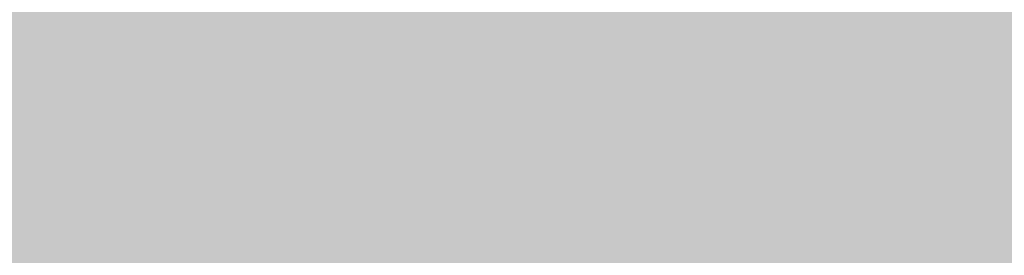
# Model space of a CAD drawing. Units: millimetres. Extents: x 0 to 2267, y 0 to 1823.
# Tile 223 of 256: x 1841.442 to 1842.748, y 1127.462 to 1127.775. Entities that reach past the tile are written whole.
import ezdxf

# ---------------------------------------------------------------- set-up
doc = ezdxf.new("R2010")
doc.units = ezdxf.units.MM
doc.header["$MEASUREMENT"] = 0
doc.layers.add('M-HATC', color=252, linetype='Continuous', lineweight=18)

msp = doc.modelspace()

# ---------------------------------------------------------------- hatches: boundary and pattern name
at = {"layer": 'M-HATC'}
h = msp.add_hatch(color=256, dxfattribs=at)
h.dxf.hatch_style = 1
h.paths.add_polyline_path([(2055.771, 1603.062), (1381.0868, 1603.062), (1381.0868, 1598.062), (2055.771, 1598.062)])
h.paths.add_polyline_path([(2055.771, 1598.062), (1381.0868, 1598.062), (1381.0868, 1593.062), (2055.771, 1593.062)])
h.paths.add_polyline_path([(2051.3074, 1536.7609), (1385.5504, 1536.7609), (1385.5504, 1526.7609), (1387.5504, 1526.7609), (1388.5366, 1525.0528), (1385.3319, 1521.2335), (1385.3319, 1521.2226), (2050.2542, 1522.7491), (2048.3212, 1525.0528), (2049.3074, 1526.7609), (2051.3074, 1526.7609)])
edge = h.paths.add_edge_path()
edge.add_arc((1847.5345, 1379.1492), 135, 222.603061, 222.890851, ccw=False)
edge.add_line((1748.1663, 1287.7656), (1683.0921, 1287.7656))
edge.add_arc((1583.7239, 1379.1492), 135, 317.109149, 317.396939, ccw=False)
edge.add_arc((1678.9686, 1290.6707), 5, 222.8909, 317.1091, ccw=False)
edge.add_arc((1774.2133, 1379.1492), 135, 222.603061, 222.890851, ccw=False)
edge.add_line((1674.8451, 1287.7656), (1609.7709, 1287.7656))
edge.add_arc((1510.4027, 1379.1492), 135, 317.109149, 317.396939, ccw=False)
edge.add_arc((1605.6474, 1290.6707), 5, 222.8909, 317.1091, ccw=False)
edge.add_arc((1700.8921, 1379.1492), 135, 222.603061, 222.890851, ccw=False)
edge.add_line((1601.5239, 1287.7656), (1536.4497, 1287.7656))
edge.add_arc((1437.0815, 1379.1492), 135, 317.109149, 317.396939, ccw=False)
edge.add_arc((1532.3262, 1290.6707), 5, 222.8909, 317.1091, ccw=False)
edge.add_arc((1627.5709, 1379.1492), 135, 222.603061, 222.890851, ccw=False)
edge.add_line((1528.2027, 1287.7656), (1505.9289, 1287.7656))
edge.add_spline(control_points=[(1505.9289, 1287.7656), (1504.2622, 1287.7656), (1504.2622, 1282.7656), (1505.9289, 1282.7656)], knot_values=[0, 0, 0, 0, 5, 5, 5, 5], degree=3, periodic=0)
edge.add_line((1505.9289, 1282.7656), (1930.9289, 1282.7656))
edge.add_spline(control_points=[(1930.9289, 1282.7656), (1932.5956, 1282.7656), (1932.5956, 1287.7656), (1930.9289, 1287.7656)], knot_values=[0, 0, 0, 0, 5, 5, 5, 5], degree=3, periodic=0)
edge.add_line((1930.9289, 1287.7656), (1903.0557, 1287.7656))
edge.add_arc((1803.6875, 1379.1492), 135, 317.109149, 317.396939, ccw=False)
edge.add_arc((1898.9322, 1290.6707), 5, 222.8909, 317.1091, ccw=False)
edge.add_arc((1994.1769, 1379.1492), 135, 222.603061, 222.890851, ccw=False)
edge.add_line((1894.8087, 1287.7656), (1829.7345, 1287.7656))
edge.add_arc((1730.3663, 1379.1492), 135, 317.109149, 317.396939, ccw=False)
edge.add_arc((1825.611, 1290.6707), 5, 222.8909, 317.1091, ccw=False)
edge.add_arc((1920.8557, 1379.1492), 135, 222.603061, 222.890851, ccw=False)
edge.add_line((1821.4875, 1287.7656), (1756.4133, 1287.7656))
edge.add_arc((1657.0451, 1379.1492), 135, 317.109149, 317.396939, ccw=False)
edge.add_arc((1752.2898, 1290.6707), 5, 222.8909, 317.1091, ccw=False)
edge = h.paths.add_edge_path()
edge.add_spline(control_points=[(1843.4289, 1227.2475), (1845.0956, 1227.2475), (1845.0956, 1232.2475), (1843.4289, 1232.2475)], knot_values=[0, 0, 0, 0, 5, 5, 5, 5], degree=3, periodic=0)
edge.add_line((1843.4289, 1232.2475), (1593.4289, 1232.2475))
edge.add_spline(control_points=[(1593.4289, 1232.2475), (1591.7622, 1232.2475), (1591.7622, 1227.2475), (1593.4289, 1227.2475)], knot_values=[0, 0, 0, 0, 5, 5, 5, 5], degree=3, periodic=0)
edge.add_line((1593.4289, 1227.2475), (1843.4289, 1227.2475))
h.paths.add_polyline_path([(1905.9289, 1127.4171), (1530.9289, 1127.4171, 0.414214), (1520.9289, 1117.4171), (1530.9289, 1117.4171), (1915.9289, 1117.4171, 0.414214)])
edge = h.paths.add_edge_path()
edge.add_arc((1397.0858, 1498.4078), 12.7299, 90.78215, 190.87871, ccw=False)
edge.add_line((1396.912, 1511.1365), (1428.0097, 1511.3488))
edge.add_line((1428.0097, 1511.3488), (1433.0097, 1511.3488))
edge.add_line((1433.0097, 1511.3488), (1434.439, 1511.3488))
edge.add_arc((1419.474, 1498.0804), 20, 41.561, 74.08211)
edge.add_line((1424.9592, 1517.3135), (1399.9351, 1517.2561))
edge.add_spline(control_points=[(1399.9307, 1517.2561), (1399.884, 1517.2131), (1399.8328, 1517.1689), (1399.7774, 1517.1236)], knot_values=[11.567499, 11.567499, 11.567499, 11.567499, 11.814249, 11.814249, 11.814249, 11.814249], degree=3, periodic=0)
edge.add_spline(control_points=[(1399.6328, 1517.0099), (1399.5831, 1516.9721), (1399.5307, 1516.9338), (1399.4759, 1516.8947)], knot_values=[11.167718, 11.167718, 11.167718, 11.167718, 11.365188, 11.365188, 11.365188, 11.365188], degree=3, periodic=0)
edge.add_spline(control_points=[(1399.3398, 1516.8001), (1399.1514, 1516.6719), (1398.9384, 1516.5377), (1398.704, 1516.3994)], knot_values=[10.376405, 10.376405, 10.376405, 10.376405, 11.00994, 11.00994, 11.00994, 11.00994], degree=3, periodic=0)
edge.add_spline(control_points=[(1398.6572, 1516.3719), (1398.5789, 1516.326), (1398.4983, 1516.2797), (1398.4155, 1516.2331)], knot_values=[10.125175, 10.125175, 10.125175, 10.125175, 10.334406, 10.334406, 10.334406, 10.334406], degree=3, periodic=0)
edge.add_spline(control_points=[(1398.2642, 1516.1487), (1398.196, 1516.1111), (1398.1263, 1516.0732), (1398.0555, 1516.0351)], knot_values=[9.832246, 9.832246, 9.832246, 9.832246, 9.999658, 9.999658, 9.999658, 9.999658], degree=3, periodic=0)
edge.add_spline(control_points=[(1397.9987, 1516.0048), (1397.7312, 1515.8621), (1397.446, 1515.7171), (1397.1466, 1515.5714)], knot_values=[9.161808, 9.161808, 9.161808, 9.161808, 9.787769, 9.787769, 9.787769, 9.787769], degree=3, periodic=0)
edge.add_spline(control_points=[(1397.1466, 1515.5714), (1396.8418, 1515.423), (1396.5222, 1515.274), (1396.1914, 1515.1262)], knot_values=[8.524455, 8.524455, 8.524455, 8.524455, 9.161808, 9.161808, 9.161808, 9.161808], degree=3, periodic=0)
edge.add_spline(control_points=[(1396.0777, 1515.0756), (1395.9854, 1515.0348), (1395.8922, 1514.994), (1395.7983, 1514.9534)], knot_values=[8.275193, 8.275193, 8.275193, 8.275193, 8.451726, 8.451726, 8.451726, 8.451726], degree=3, periodic=0)
edge.add_spline(control_points=[(1395.6018, 1514.8691), (1395.4997, 1514.8257), (1395.3968, 1514.7824), (1395.2932, 1514.7394)], knot_values=[7.962917, 7.962917, 7.962917, 7.962917, 8.152764, 8.152764, 8.152764, 8.152764], degree=3, periodic=0)
edge.add_spline(control_points=[(1395.2116, 1514.7057), (1394.8278, 1514.5475), (1394.4345, 1514.3929), (1394.0364, 1514.2442)], knot_values=[7.21254, 7.21254, 7.21254, 7.21254, 7.913148, 7.913148, 7.913148, 7.913148], degree=3, periodic=0)
edge.add_spline(control_points=[(1394.0364, 1514.2442), (1393.7076, 1514.1214), (1393.3754, 1514.0027), (1393.0427, 1513.8895)], knot_values=[6.633733, 6.633733, 6.633733, 6.633733, 7.21254, 7.21254, 7.21254, 7.21254], degree=3, periodic=0)
edge.add_spline(control_points=[(1392.8214, 1513.815), (1392.7198, 1513.7812), (1392.6181, 1513.7479), (1392.5166, 1513.7152)], knot_values=[6.328796, 6.328796, 6.328796, 6.328796, 6.505493, 6.505493, 6.505493, 6.505493], degree=3, periodic=0)
edge.add_spline(control_points=[(1392.5166, 1513.7152), (1392.3187, 1513.6515), (1392.1212, 1513.59), (1391.9244, 1513.531)], knot_values=[5.984605, 5.984605, 5.984605, 5.984605, 6.328796, 6.328796, 6.328796, 6.328796], degree=3, periodic=0)
edge.add_spline(control_points=[(1391.7915, 1513.4915), (1391.3122, 1513.3501), (1390.8384, 1513.2239), (1390.3784, 1513.1171)], knot_values=[5.066697, 5.066697, 5.066697, 5.066697, 5.907055, 5.907055, 5.907055, 5.907055], degree=3, periodic=0)
edge.add_spline(control_points=[(1390.3784, 1513.1171), (1390.1797, 1513.071), (1389.9836, 1513.0284), (1389.7907, 1512.9899)], knot_values=[4.70367, 4.70367, 4.70367, 4.70367, 5.066695, 5.066695, 5.066695, 5.066695], degree=3, periodic=0)
edge.add_spline(control_points=[(1389.422, 1512.9204), (1389.2459, 1512.8892), (1389.0729, 1512.8617), (1388.9036, 1512.8381)], knot_values=[4.130571, 4.130571, 4.130571, 4.130571, 4.469816, 4.469816, 4.469816, 4.469816], degree=3, periodic=0)
edge.add_spline(control_points=[(1388.9036, 1512.8381), (1388.591, 1512.7946), (1388.2911, 1512.7644), (1388.0071, 1512.7494)], knot_values=[3.504031, 3.504031, 3.504031, 3.504031, 4.130571, 4.130571, 4.130571, 4.130571], degree=3, periodic=0)
edge.add_spline(control_points=[(1387.9356, 1512.7459), (1387.8538, 1512.7423), (1387.7733, 1512.74), (1387.6944, 1512.739)], knot_values=[3.268866, 3.268866, 3.268866, 3.268866, 3.451164, 3.451164, 3.451164, 3.451164], degree=3, periodic=0)
edge.add_spline(control_points=[(1387.3351, 1512.7443), (1387.2076, 1512.7499), (1387.0847, 1512.7597), (1386.967, 1512.7739)], knot_values=[2.670686, 2.670686, 2.670686, 2.670686, 2.984, 2.984, 2.984, 2.984], degree=3, periodic=0)
edge.add_spline(control_points=[(1386.8327, 1512.7922), (1386.8209, 1512.7941), (1386.8092, 1512.7959), (1386.7975, 1512.7979)], knot_values=[2.516981, 2.516981, 2.516981, 2.516981, 2.549528, 2.549528, 2.549528, 2.549528], degree=3, periodic=0)
edge.add_spline(control_points=[(1386.4526, 1512.8735), (1386.4257, 1512.881), (1386.3993, 1512.889), (1386.3733, 1512.8972)], knot_values=[2.095869, 2.095869, 2.095869, 2.095869, 2.17941, 2.17941, 2.17941, 2.17941], degree=3, periodic=0)
edge.add_spline(control_points=[(1386.0691, 1513.0189), (1386.0634, 1513.0217), (1386.0577, 1513.0246), (1386.052, 1513.0275)], knot_values=[1.72453, 1.72453, 1.72453, 1.72453, 1.745933, 1.745933, 1.745933, 1.745933], degree=3, periodic=0)
edge.add_arc((1399.474, 1498.0804), 20, 131.82432, 180)
edge.add_arc((1630.3336, 1505.5484), 250.9708, 181.705176, 236.427975)
edge.add_arc((1605.3399, 1483.3044), 218.7822, 238.660829, 243.34961)
edge.add_arc((1647.0911, 1510.3592), 262.8986, 183.129836, 237.853442, ccw=False)
h.paths.add_polyline_path([(1406.5369, 1391.9644, 0.149382), (1491.5506, 1296.4418, -0.129517)], flags=17)
edge = h.paths.add_edge_path()
edge.add_arc((2037.3838, 1498.0804), 20, 0, 48.26587)
edge.add_spline(control_points=[(2050.6973, 1513.0052), (2050.6512, 1512.9847), (2050.6034, 1512.9655), (2050.5539, 1512.9477)], knot_values=[1.835652, 1.835652, 1.835652, 1.835652, 2.000781, 2.000781, 2.000781, 2.000781], degree=3, periodic=0)
edge.add_spline(control_points=[(2050.4616, 1512.9166), (2050.479, 1512.9221), (2050.4963, 1512.9277), (2050.5133, 1512.9335)], knot_values=[2.045477, 2.045477, 2.045477, 2.045477, 2.101389, 2.101389, 2.101389, 2.101389], degree=3, periodic=0)
edge.add_spline(control_points=[(2050.129, 1512.8342), (2050.1984, 1512.8473), (2050.2657, 1512.8623), (2050.3308, 1512.8792)], knot_values=[2.237629, 2.237629, 2.237629, 2.237629, 2.435841, 2.435841, 2.435841, 2.435841], degree=3, periodic=0)
edge.add_spline(control_points=[(2050.0946, 1512.8278), (2050.1061, 1512.8299), (2050.1176, 1512.832), (2050.129, 1512.8342)], knot_values=[2.435841, 2.435841, 2.435841, 2.435841, 2.468321, 2.468321, 2.468321, 2.468321], degree=3, periodic=0)
edge.add_spline(control_points=[(2049.7843, 1512.7851), (2049.8552, 1512.7922), (2049.9243, 1512.8008), (2049.9917, 1512.8109)], knot_values=[2.563852, 2.563852, 2.563852, 2.563852, 2.748541, 2.748541, 2.748541, 2.748541], degree=3, periodic=0)
edge.add_spline(control_points=[(2049.4052, 1512.7617), (2049.5364, 1512.7653), (2049.6629, 1512.773), (2049.7843, 1512.7851)], knot_values=[2.748541, 2.748541, 2.748541, 2.748541, 3.064882, 3.064882, 3.064882, 3.064882], degree=3, periodic=0)
edge.add_spline(control_points=[(2049.1698, 1512.7597), (2049.2336, 1512.7591), (2049.2965, 1512.7594), (2049.3584, 1512.7606)], knot_values=[3.102309, 3.102309, 3.102309, 3.102309, 3.2503, 3.2503, 3.2503, 3.2503], degree=3, periodic=0)
edge.add_spline(control_points=[(2048.8573, 1512.7691), (2048.9638, 1512.7638), (2049.068, 1512.7606), (2049.1698, 1512.7597)], knot_values=[3.2503, 3.2503, 3.2503, 3.2503, 3.486069, 3.486069, 3.486069, 3.486069], degree=3, periodic=0)
edge.add_spline(control_points=[(2048.6924, 1512.7789), (2048.3729, 1512.8009), (2048.0345, 1512.8411), (2047.6817, 1512.897)], knot_values=[3.606429, 3.606429, 3.606429, 3.606429, 4.2989, 4.2989, 4.2989, 4.2989], degree=3, periodic=0)
edge.add_spline(control_points=[(2047.6817, 1512.897), (2047.5458, 1512.9185), (2047.4077, 1512.9424), (2047.2678, 1512.9685)], knot_values=[4.2989, 4.2989, 4.2989, 4.2989, 4.565769, 4.565769, 4.565769, 4.565769], degree=3, periodic=0)
edge.add_spline(control_points=[(2047.2678, 1512.9685), (2047.1449, 1512.9914), (2047.0207, 1513.016), (2046.8951, 1513.0422)], knot_values=[4.565769, 4.565769, 4.565769, 4.565769, 4.799971, 4.799971, 4.799971, 4.799971], degree=3, periodic=0)
edge.add_spline(control_points=[(2046.8951, 1513.0422), (2046.5286, 1513.1188), (2046.1513, 1513.209), (2045.7676, 1513.3107)], knot_values=[4.799971, 4.799971, 4.799971, 4.799971, 5.483718, 5.483718, 5.483718, 5.483718], degree=3, periodic=0)
edge.add_spline(control_points=[(2045.7676, 1513.3107), (2045.3724, 1513.4154), (2044.9704, 1513.5322), (2044.5662, 1513.6588)], knot_values=[5.483718, 5.483718, 5.483718, 5.483718, 6.187866, 6.187866, 6.187866, 6.187866], degree=3, periodic=0)
edge.add_spline(control_points=[(2044.5662, 1513.6588), (2044.4149, 1513.7061), (2044.2633, 1513.7549), (2044.1116, 1513.8048)], knot_values=[6.187866, 6.187866, 6.187866, 6.187866, 6.451551, 6.451551, 6.451551, 6.451551], degree=3, periodic=0)
edge.add_spline(control_points=[(2044.1116, 1513.8048), (2043.9967, 1513.8427), (2043.8817, 1513.8813), (2043.7668, 1513.9205)], knot_values=[6.451551, 6.451551, 6.451551, 6.451551, 6.651434, 6.651434, 6.651434, 6.651434], degree=3, periodic=0)
edge.add_spline(control_points=[(2043.7668, 1513.9205), (2043.3716, 1514.0554), (2042.9774, 1514.1979), (2042.5886, 1514.3458)], knot_values=[6.651434, 6.651434, 6.651434, 6.651434, 7.338879, 7.338879, 7.338879, 7.338879], degree=3, periodic=0)
edge.add_spline(control_points=[(2042.5886, 1514.3458), (2042.1643, 1514.5071), (2041.7465, 1514.6749), (2041.3409, 1514.846)], knot_values=[7.338879, 7.338879, 7.338879, 7.338879, 8.089209, 8.089209, 8.089209, 8.089209], degree=3, periodic=0)
edge.add_spline(control_points=[(2041.3409, 1514.846), (2041.1028, 1514.9465), (2040.869, 1515.0481), (2040.6405, 1515.1502)], knot_values=[8.089209, 8.089209, 8.089209, 8.089209, 8.529587, 8.529587, 8.529587, 8.529587], degree=3, periodic=0)
edge.add_spline(control_points=[(2040.51, 1515.2089), (2040.0824, 1515.4022), (2039.6747, 1515.5971), (2039.295, 1515.7894)], knot_values=[8.613818, 8.613818, 8.613818, 8.613818, 9.44571, 9.44571, 9.44571, 9.44571], degree=3, periodic=0)
edge.add_spline(control_points=[(2039.295, 1515.7894), (2039.0618, 1515.9075), (2038.8391, 1516.0246), (2038.6288, 1516.1398)], knot_values=[9.44571, 9.44571, 9.44571, 9.44571, 9.956404, 9.956404, 9.956404, 9.956404], degree=3, periodic=0)
edge.add_spline(control_points=[(2038.6288, 1516.1398), (2038.5187, 1516.2001), (2038.4121, 1516.2598), (2038.309, 1516.3189)], knot_values=[9.956404, 9.956404, 9.956404, 9.956404, 10.223542, 10.223542, 10.223542, 10.223542], degree=3, periodic=0)
edge.add_spline(control_points=[(2038.309, 1516.3189), (2038.2138, 1516.3735), (2038.1216, 1516.4276), (2038.0328, 1516.481)], knot_values=[10.223542, 10.223542, 10.223542, 10.223542, 10.47051, 10.47051, 10.47051, 10.47051], degree=3, periodic=0)
edge.add_spline(control_points=[(2038.0328, 1516.481), (2037.7855, 1516.6296), (2037.5639, 1516.773), (2037.3722, 1516.909)], knot_values=[10.47051, 10.47051, 10.47051, 10.47051, 11.15767, 11.15767, 11.15767, 11.15767], degree=3, periodic=0)
edge.add_spline(control_points=[(2037.3722, 1516.909), (2037.2789, 1516.9752), (2037.1927, 1517.0396), (2037.1142, 1517.102)], knot_values=[11.15767, 11.15767, 11.15767, 11.15767, 11.49227, 11.49227, 11.49227, 11.49227], degree=3, periodic=0)
edge.add_spline(control_points=[(2036.8564, 1517.3259), (2036.9148, 1517.2692), (2036.9814, 1517.2103), (2037.0557, 1517.1492)], knot_values=[11.577341, 11.577341, 11.577341, 11.577341, 11.91035, 11.91035, 11.91035, 11.91035], degree=3, periodic=0)
edge.add_spline(control_points=[(2036.8074, 1517.3748), (2036.823, 1517.3587), (2036.8393, 1517.3424), (2036.8564, 1517.3259)], knot_values=[11.91035, 11.91035, 11.91035, 11.91035, 12.007402, 12.007402, 12.007402, 12.007402], degree=3, periodic=0)
edge.add_spline(control_points=[(2036.7017, 1517.494), (2036.7104, 1517.483), (2036.7196, 1517.4719), (2036.7291, 1517.4606)], knot_values=[12.184155, 12.184155, 12.184155, 12.184155, 12.255409, 12.255409, 12.255409, 12.255409], degree=3, periodic=0)
edge.add_spline(control_points=[(2036.6159, 1517.6205), (2036.62, 1517.613), (2036.6243, 1517.6055), (2036.6289, 1517.5979)], knot_values=[12.487913, 12.487913, 12.487913, 12.487913, 12.541035, 12.541035, 12.541035, 12.541035], degree=3, periodic=0)
edge.add_spline(control_points=[(2036.5635, 1517.786), (2036.5637, 1517.7794), (2036.5642, 1517.7726), (2036.565, 1517.7658)], knot_values=[12.911761, 12.911761, 12.911761, 12.911761, 12.968286, 12.968286, 12.968286, 12.968286], degree=3, periodic=0)
edge.add_spline(control_points=[(2036.6166, 1517.9304), (2036.6125, 1517.9259), (2036.6086, 1517.9212), (2036.6049, 1517.9165)], knot_values=[13.382527, 13.382527, 13.382527, 13.382527, 13.433791, 13.433791, 13.433791, 13.433791], degree=3, periodic=0)
edge.add_spline(control_points=[(2036.749, 1518.017), (2036.7361, 1518.0116), (2036.7239, 1518.006), (2036.7124, 1518.0002)], knot_values=[13.726299, 13.726299, 13.726299, 13.726299, 13.809928, 13.809928, 13.809928, 13.809928], degree=3, periodic=0)
edge.add_spline(control_points=[(2036.8604, 1518.0528), (2036.8386, 1518.0474), (2036.8181, 1518.0416), (2036.7988, 1518.0353)], knot_values=[13.910887, 13.910887, 13.910887, 13.910887, 14.02153, 14.02153, 14.02153, 14.02153], degree=3, periodic=0)
edge.add_line((2036.9639, 1518.0804), (2032.3838, 1518.0804))
edge.add_line((2032.3838, 1518.0804), (2027.3838, 1518.0804))
edge.add_line((2027.3838, 1518.0804), (2022.3838, 1518.0804))
edge.add_line((2022.3838, 1518.0804), (2017.3838, 1518.0804))
edge.add_arc((2017.3838, 1498.0804), 20, 90, 138.439)
edge.add_line((2002.4188, 1511.3488), (2003.8481, 1511.3488))
edge.add_line((2003.8481, 1511.3488), (2008.8481, 1511.3488))
edge.add_line((2008.8481, 1511.3488), (2039.772, 1511.1377))
edge.add_arc((2039.772, 1498.4078), 12.7299, -10.87871, 90, ccw=False)
edge.add_arc((1789.7668, 1510.3592), 262.8986, 302.146558, 356.870164, ccw=False)
edge.add_arc((1831.5179, 1483.3044), 218.7822, 296.65039, 301.339171)
edge.add_arc((1806.5242, 1505.5484), 250.9708, 303.572025, 358.294824)
h.paths.add_polyline_path([(2030.321, 1391.9644, -0.129517), (1945.3072, 1296.4418, 0.149382)], flags=17)
edge = h.paths.add_edge_path()
edge.add_spline(control_points=[(2037.2464, 1518.0821), (2037.2898, 1518.081), (2037.3355, 1518.0804), (2037.3838, 1518.0804)], knot_values=[0.000012, 0.000012, 0.000012, 0.000012, 0.144754, 0.144754, 0.144754, 0.144754], degree=3, periodic=0)
edge.add_line((2037.3357, 1518.0804), (2037.0096, 1518.0804))
edge.add_spline(control_points=[(2037.0096, 1518.0804), (2036.9822, 1518.0768), (2036.956, 1518.0727), (2036.9312, 1518.0681)], knot_values=[14.13465, 14.13465, 14.13465, 14.13465, 14.247197, 14.247197, 14.247197, 14.247197], degree=3, periodic=0)
edge.add_spline(control_points=[(2036.9312, 1518.0681), (2036.9276, 1518.0674), (2036.9241, 1518.0667), (2036.9205, 1518.0661)], knot_values=[14.118315, 14.118315, 14.118315, 14.118315, 14.13465, 14.13465, 14.13465, 14.13465], degree=3, periodic=0)
edge.add_spline(control_points=[(2036.9205, 1518.0661), (2036.9118, 1518.0644), (2036.9032, 1518.0626), (2036.8948, 1518.0608)], knot_values=[14.078086, 14.078086, 14.078086, 14.078086, 14.118315, 14.118315, 14.118315, 14.118315], degree=3, periodic=0)
edge.add_spline(control_points=[(2036.8948, 1518.0608), (2036.883, 1518.0583), (2036.8716, 1518.0556), (2036.8604, 1518.0528)], knot_values=[14.02153, 14.02153, 14.02153, 14.02153, 14.078086, 14.078086, 14.078086, 14.078086], degree=3, periodic=0)
edge.add_spline(control_points=[(2036.8604, 1518.0528), (2036.8386, 1518.0474), (2036.8181, 1518.0416), (2036.7988, 1518.0353)], knot_values=[13.910887, 13.910887, 13.910887, 13.910887, 14.02153, 14.02153, 14.02153, 14.02153], degree=3, periodic=0)
edge.add_spline(control_points=[(2036.7988, 1518.0353), (2036.7981, 1518.035), (2036.7974, 1518.0348), (2036.7967, 1518.0346)], knot_values=[13.906906, 13.906906, 13.906906, 13.906906, 13.910887, 13.910887, 13.910887, 13.910887], degree=3, periodic=0)
edge.add_spline(control_points=[(2036.7967, 1518.0346), (2036.7882, 1518.0318), (2036.7799, 1518.0289), (2036.7719, 1518.0259)], knot_values=[13.857826, 13.857826, 13.857826, 13.857826, 13.906906, 13.906906, 13.906906, 13.906906], degree=3, periodic=0)
edge.add_spline(control_points=[(2036.7719, 1518.0259), (2036.764, 1518.023), (2036.7564, 1518.02), (2036.749, 1518.017)], knot_values=[13.809928, 13.809928, 13.809928, 13.809928, 13.857826, 13.857826, 13.857826, 13.857826], degree=3, periodic=0)
edge.add_spline(control_points=[(2036.749, 1518.017), (2036.7361, 1518.0116), (2036.7239, 1518.006), (2036.7124, 1518.0002)], knot_values=[13.726299, 13.726299, 13.726299, 13.726299, 13.809928, 13.809928, 13.809928, 13.809928], degree=3, periodic=0)
edge.add_spline(control_points=[(2036.7124, 1518.0002), (2036.7121, 1518), (2036.7118, 1517.9999), (2036.7115, 1517.9997)], knot_values=[13.723993, 13.723993, 13.723993, 13.723993, 13.726299, 13.726299, 13.726299, 13.726299], degree=3, periodic=0)
edge.add_spline(control_points=[(2036.7115, 1517.9997), (2036.7063, 1517.9971), (2036.7013, 1517.9944), (2036.6965, 1517.9917)], knot_values=[13.686536, 13.686536, 13.686536, 13.686536, 13.723993, 13.723993, 13.723993, 13.723993], degree=3, periodic=0)
edge.add_spline(control_points=[(2036.6965, 1517.9917), (2036.6919, 1517.9891), (2036.6874, 1517.9865), (2036.6831, 1517.9839)], knot_values=[13.651251, 13.651251, 13.651251, 13.651251, 13.686536, 13.686536, 13.686536, 13.686536], degree=3, periodic=0)
edge.add_spline(control_points=[(2036.6831, 1517.9839), (2036.6764, 1517.9798), (2036.67, 1517.9757), (2036.6639, 1517.9714)], knot_values=[13.596804, 13.596804, 13.596804, 13.596804, 13.651251, 13.651251, 13.651251, 13.651251], degree=3, periodic=0)
edge.add_spline(control_points=[(2036.6639, 1517.9714), (2036.6636, 1517.9712), (2036.6633, 1517.9709), (2036.6629, 1517.9707)], knot_values=[13.593956, 13.593956, 13.593956, 13.593956, 13.596804, 13.596804, 13.596804, 13.596804], degree=3, periodic=0)
edge.add_spline(control_points=[(2036.6629, 1517.9707), (2036.6603, 1517.9689), (2036.6577, 1517.967), (2036.6552, 1517.9651)], knot_values=[13.570322, 13.570322, 13.570322, 13.570322, 13.593956, 13.593956, 13.593956, 13.593956], degree=3, periodic=0)
edge.add_spline(control_points=[(2036.6552, 1517.9651), (2036.6525, 1517.9631), (2036.6499, 1517.9611), (2036.6474, 1517.9591)], knot_values=[13.545477, 13.545477, 13.545477, 13.545477, 13.570322, 13.570322, 13.570322, 13.570322], degree=3, periodic=0)
edge.add_spline(control_points=[(2036.6474, 1517.9591), (2036.6472, 1517.9589), (2036.6471, 1517.9588), (2036.6469, 1517.9587)], knot_values=[13.543931, 13.543931, 13.543931, 13.543931, 13.545477, 13.545477, 13.545477, 13.545477], degree=3, periodic=0)
edge.add_spline(control_points=[(2036.6469, 1517.9587), (2036.6412, 1517.9541), (2036.6358, 1517.9494), (2036.6307, 1517.9447)], knot_values=[13.488237, 13.488237, 13.488237, 13.488237, 13.543931, 13.543931, 13.543931, 13.543931], degree=3, periodic=0)
edge.add_spline(control_points=[(2036.6307, 1517.9447), (2036.6282, 1517.9423), (2036.6257, 1517.9399), (2036.6233, 1517.9374)], knot_values=[13.460307, 13.460307, 13.460307, 13.460307, 13.488237, 13.488237, 13.488237, 13.488237], degree=3, periodic=0)
edge.add_spline(control_points=[(2036.6233, 1517.9374), (2036.6215, 1517.9356), (2036.6198, 1517.9338), (2036.6181, 1517.932)], knot_values=[13.439712, 13.439712, 13.439712, 13.439712, 13.460307, 13.460307, 13.460307, 13.460307], degree=3, periodic=0)
edge.add_spline(control_points=[(2036.6181, 1517.932), (2036.6176, 1517.9315), (2036.6171, 1517.9309), (2036.6166, 1517.9304)], knot_values=[13.433791, 13.433791, 13.433791, 13.433791, 13.439712, 13.439712, 13.439712, 13.439712], degree=3, periodic=0)
edge.add_spline(control_points=[(2036.6166, 1517.9304), (2036.6125, 1517.9259), (2036.6086, 1517.9212), (2036.6049, 1517.9165)], knot_values=[13.382527, 13.382527, 13.382527, 13.382527, 13.433791, 13.433791, 13.433791, 13.433791], degree=3, periodic=0)
edge.add_spline(control_points=[(2036.6049, 1517.9165), (2036.6026, 1517.9135), (2036.6004, 1517.9104), (2036.5982, 1517.9074)], knot_values=[13.350017, 13.350017, 13.350017, 13.350017, 13.382527, 13.382527, 13.382527, 13.382527], degree=3, periodic=0)
edge.add_spline(control_points=[(2036.5982, 1517.9074), (2036.5972, 1517.9059), (2036.5962, 1517.9043), (2036.5952, 1517.9028)], knot_values=[13.333922, 13.333922, 13.333922, 13.333922, 13.350017, 13.350017, 13.350017, 13.350017], degree=3, periodic=0)
edge.add_spline(control_points=[(2036.5952, 1517.9028), (2036.5945, 1517.9018), (2036.5939, 1517.9009), (2036.5933, 1517.8999)], knot_values=[13.323828, 13.323828, 13.323828, 13.323828, 13.333922, 13.333922, 13.333922, 13.333922], degree=3, periodic=0)
edge.add_spline(control_points=[(2036.5933, 1517.8999), (2036.5905, 1517.8955), (2036.5879, 1517.8909), (2036.5855, 1517.8864)], knot_values=[13.277545, 13.277545, 13.277545, 13.277545, 13.323828, 13.323828, 13.323828, 13.323828], degree=3, periodic=0)
edge.add_spline(control_points=[(2036.5855, 1517.8864), (2036.5836, 1517.8827), (2036.5817, 1517.8789), (2036.5801, 1517.8751)], knot_values=[13.240119, 13.240119, 13.240119, 13.240119, 13.277545, 13.277545, 13.277545, 13.277545], degree=3, periodic=0)
edge.add_spline(control_points=[(2036.5801, 1517.8751), (2036.5795, 1517.8739), (2036.579, 1517.8727), (2036.5785, 1517.8715)], knot_values=[13.228211, 13.228211, 13.228211, 13.228211, 13.240119, 13.240119, 13.240119, 13.240119], degree=3, periodic=0)
edge.add_spline(control_points=[(2036.5785, 1517.8715), (2036.578, 1517.8702), (2036.5774, 1517.869), (2036.5769, 1517.8677)], knot_values=[13.215717, 13.215717, 13.215717, 13.215717, 13.228211, 13.228211, 13.228211, 13.228211], degree=3, periodic=0)
edge.add_spline(control_points=[(2036.5769, 1517.8677), (2036.5755, 1517.864), (2036.5741, 1517.8603), (2036.5729, 1517.8565)], knot_values=[13.179847, 13.179847, 13.179847, 13.179847, 13.215717, 13.215717, 13.215717, 13.215717], degree=3, periodic=0)
edge.add_spline(control_points=[(2036.5729, 1517.8565), (2036.5713, 1517.8515), (2036.5699, 1517.8464), (2036.5687, 1517.8413)], knot_values=[13.132017, 13.132017, 13.132017, 13.132017, 13.179847, 13.179847, 13.179847, 13.179847], degree=3, periodic=0)
edge.add_spline(control_points=[(2036.5687, 1517.8413), (2036.5684, 1517.8402), (2036.5682, 1517.8392), (2036.568, 1517.8382)], knot_values=[13.122482, 13.122482, 13.122482, 13.122482, 13.132017, 13.132017, 13.132017, 13.132017], degree=3, periodic=0)
edge.add_spline(control_points=[(2036.568, 1517.8382), (2036.5676, 1517.8363), (2036.5672, 1517.8345), (2036.5669, 1517.8327)], knot_values=[13.105592, 13.105592, 13.105592, 13.105592, 13.122482, 13.122482, 13.122482, 13.122482], degree=3, periodic=0)
edge.add_spline(control_points=[(2036.5669, 1517.8327), (2036.5662, 1517.8292), (2036.5657, 1517.8257), (2036.5652, 1517.8222)], knot_values=[13.074063, 13.074063, 13.074063, 13.074063, 13.105592, 13.105592, 13.105592, 13.105592], degree=3, periodic=0)
edge.add_spline(control_points=[(2036.5652, 1517.8222), (2036.5652, 1517.8222), (2036.5652, 1517.8222), (2036.5652, 1517.8222)], knot_values=[13.074043, 13.074043, 13.074043, 13.074043, 13.074063, 13.074063, 13.074063, 13.074063], degree=3, periodic=0)
edge.add_spline(control_points=[(2036.5652, 1517.8222), (2036.5644, 1517.8164), (2036.5639, 1517.8106), (2036.5636, 1517.8046)], knot_values=[13.021884, 13.021884, 13.021884, 13.021884, 13.074043, 13.074043, 13.074043, 13.074043], degree=3, periodic=0)
edge.add_spline(control_points=[(2036.5636, 1517.8046), (2036.5636, 1517.804), (2036.5636, 1517.8034), (2036.5635, 1517.8028)], knot_values=[13.01674, 13.01674, 13.01674, 13.01674, 13.021884, 13.021884, 13.021884, 13.021884], degree=3, periodic=0)
edge.add_spline(control_points=[(2036.5635, 1517.8028), (2036.5634, 1517.8005), (2036.5634, 1517.7982), (2036.5634, 1517.7958)], knot_values=[12.996438, 12.996438, 12.996438, 12.996438, 13.01674, 13.01674, 13.01674, 13.01674], degree=3, periodic=0)
edge.add_spline(control_points=[(2036.5634, 1517.7958), (2036.5633, 1517.7926), (2036.5634, 1517.7893), (2036.5635, 1517.786)], knot_values=[12.968286, 12.968286, 12.968286, 12.968286, 12.996438, 12.996438, 12.996438, 12.996438], degree=3, periodic=0)
edge.add_spline(control_points=[(2036.5635, 1517.786), (2036.5637, 1517.7794), (2036.5642, 1517.7726), (2036.565, 1517.7658)], knot_values=[12.911761, 12.911761, 12.911761, 12.911761, 12.968286, 12.968286, 12.968286, 12.968286], degree=3, periodic=0)
edge.add_spline(control_points=[(2036.565, 1517.7658), (2036.565, 1517.7657), (2036.565, 1517.7656), (2036.565, 1517.7656)], knot_values=[12.911017, 12.911017, 12.911017, 12.911017, 12.911761, 12.911761, 12.911761, 12.911761], degree=3, periodic=0)
edge.add_spline(control_points=[(2036.565, 1517.7656), (2036.5654, 1517.7625), (2036.5658, 1517.7593), (2036.5663, 1517.7562)], knot_values=[12.88528, 12.88528, 12.88528, 12.88528, 12.911017, 12.911017, 12.911017, 12.911017], degree=3, periodic=0)
edge.add_spline(control_points=[(2036.5663, 1517.7562), (2036.5667, 1517.7534), (2036.5672, 1517.7506), (2036.5677, 1517.7478)], knot_values=[12.862519, 12.862519, 12.862519, 12.862519, 12.88528, 12.88528, 12.88528, 12.88528], degree=3, periodic=0)
edge.add_spline(control_points=[(2036.5677, 1517.7478), (2036.5678, 1517.7474), (2036.5679, 1517.7469), (2036.568, 1517.7465)], knot_values=[12.858885, 12.858885, 12.858885, 12.858885, 12.862519, 12.862519, 12.862519, 12.862519], degree=3, periodic=0)
edge.add_spline(control_points=[(2036.568, 1517.7465), (2036.5692, 1517.7399), (2036.5707, 1517.7332), (2036.5724, 1517.7264)], knot_values=[12.8053, 12.8053, 12.8053, 12.8053, 12.858885, 12.858885, 12.858885, 12.858885], degree=3, periodic=0)
edge.add_spline(control_points=[(2036.5724, 1517.7264), (2036.5734, 1517.7226), (2036.5745, 1517.7187), (2036.5756, 1517.7149)], knot_values=[12.775176, 12.775176, 12.775176, 12.775176, 12.8053, 12.8053, 12.8053, 12.8053], degree=3, periodic=0)
edge.add_spline(control_points=[(2036.5756, 1517.7149), (2036.5763, 1517.7125), (2036.577, 1517.7102), (2036.5778, 1517.7078)], knot_values=[12.756759, 12.756759, 12.756759, 12.756759, 12.775176, 12.775176, 12.775176, 12.775176], degree=3, periodic=0)
edge.add_spline(control_points=[(2036.5778, 1517.7078), (2036.5781, 1517.7067), (2036.5784, 1517.7057), (2036.5787, 1517.7047)], knot_values=[12.748742, 12.748742, 12.748742, 12.748742, 12.756759, 12.756759, 12.756759, 12.756759], degree=3, periodic=0)
edge.add_spline(control_points=[(2036.5787, 1517.7047), (2036.5808, 1517.6983), (2036.5831, 1517.6919), (2036.5856, 1517.6854)], knot_values=[12.69959, 12.69959, 12.69959, 12.69959, 12.748742, 12.748742, 12.748742, 12.748742], degree=3, periodic=0)
edge.add_spline(control_points=[(2036.5856, 1517.6854), (2036.5876, 1517.68), (2036.5898, 1517.6746), (2036.5921, 1517.6692)], knot_values=[12.659038, 12.659038, 12.659038, 12.659038, 12.69959, 12.69959, 12.69959, 12.69959], degree=3, periodic=0)
edge.add_spline(control_points=[(2036.5921, 1517.6692), (2036.594, 1517.6648), (2036.5959, 1517.6605), (2036.5979, 1517.6561)], knot_values=[12.626806, 12.626806, 12.626806, 12.626806, 12.659038, 12.659038, 12.659038, 12.659038], degree=3, periodic=0)
edge.add_spline(control_points=[(2036.5979, 1517.6561), (2036.5984, 1517.6551), (2036.5989, 1517.6541), (2036.5993, 1517.6531)], knot_values=[12.619394, 12.619394, 12.619394, 12.619394, 12.626806, 12.626806, 12.626806, 12.626806], degree=3, periodic=0)
edge.add_spline(control_points=[(2036.5993, 1517.6531), (2036.6043, 1517.6424), (2036.6099, 1517.6315), (2036.6159, 1517.6205)], knot_values=[12.541039, 12.541039, 12.541039, 12.541039, 12.619394, 12.619394, 12.619394, 12.619394], degree=3, periodic=0)
edge.add_spline(control_points=[(2036.6159, 1517.6205), (2036.6159, 1517.6205), (2036.6159, 1517.6205), (2036.6159, 1517.6205)], knot_values=[12.541035, 12.541035, 12.541035, 12.541035, 12.541039, 12.541039, 12.541039, 12.541039], degree=3, periodic=0)
edge.add_spline(control_points=[(2036.6159, 1517.6205), (2036.62, 1517.613), (2036.6243, 1517.6055), (2036.6289, 1517.5979)], knot_values=[12.487913, 12.487913, 12.487913, 12.487913, 12.541035, 12.541035, 12.541035, 12.541035], degree=3, periodic=0)
edge.add_spline(control_points=[(2036.6289, 1517.5979), (2036.6326, 1517.5916), (2036.6365, 1517.5853), (2036.6406, 1517.5789)], knot_values=[12.443982, 12.443982, 12.443982, 12.443982, 12.487913, 12.487913, 12.487913, 12.487913], degree=3, periodic=0)
edge.add_spline(control_points=[(2036.6406, 1517.5789), (2036.6414, 1517.5776), (2036.6423, 1517.5763), (2036.6431, 1517.5749)], knot_values=[12.434996, 12.434996, 12.434996, 12.434996, 12.443982, 12.443982, 12.443982, 12.443982], degree=3, periodic=0)
edge.add_spline(control_points=[(2036.6431, 1517.5749), (2036.6531, 1517.5596), (2036.6639, 1517.5439), (2036.6756, 1517.528)], knot_values=[12.329647, 12.329647, 12.329647, 12.329647, 12.434996, 12.434996, 12.434996, 12.434996], degree=3, periodic=0)
edge.add_spline(control_points=[(2036.6756, 1517.528), (2036.6839, 1517.5168), (2036.6925, 1517.5055), (2036.7017, 1517.494)], knot_values=[12.255409, 12.255409, 12.255409, 12.255409, 12.329647, 12.329647, 12.329647, 12.329647], degree=3, periodic=0)
edge.add_spline(control_points=[(2036.7017, 1517.494), (2036.7104, 1517.483), (2036.7196, 1517.4719), (2036.7291, 1517.4606)], knot_values=[12.184155, 12.184155, 12.184155, 12.184155, 12.255409, 12.255409, 12.255409, 12.255409], degree=3, periodic=0)
edge.add_spline(control_points=[(2036.7291, 1517.4606), (2036.7436, 1517.4435), (2036.759, 1517.4262), (2036.7753, 1517.4085)], knot_values=[12.075961, 12.075961, 12.075961, 12.075961, 12.184155, 12.184155, 12.184155, 12.184155], degree=3, periodic=0)
edge.add_spline(control_points=[(2036.7753, 1517.4085), (2036.7763, 1517.4075), (2036.7773, 1517.4064), (2036.7783, 1517.4054)], knot_values=[12.069502, 12.069502, 12.069502, 12.069502, 12.075961, 12.075961, 12.075961, 12.075961], degree=3, periodic=0)
edge.add_spline(control_points=[(2036.7783, 1517.4054), (2036.7877, 1517.3953), (2036.7974, 1517.385), (2036.8074, 1517.3748)], knot_values=[12.007402, 12.007402, 12.007402, 12.007402, 12.069502, 12.069502, 12.069502, 12.069502], degree=3, periodic=0)
edge.add_spline(control_points=[(2036.8074, 1517.3748), (2036.823, 1517.3587), (2036.8393, 1517.3424), (2036.8564, 1517.3259)], knot_values=[11.91035, 11.91035, 11.91035, 11.91035, 12.007402, 12.007402, 12.007402, 12.007402], degree=3, periodic=0)
edge.add_spline(control_points=[(2036.8564, 1517.3259), (2036.9148, 1517.2692), (2036.9814, 1517.2103), (2037.0557, 1517.1492)], knot_values=[11.577341, 11.577341, 11.577341, 11.577341, 11.91035, 11.91035, 11.91035, 11.91035], degree=3, periodic=0)
edge.add_spline(control_points=[(2037.0557, 1517.1492), (2037.0747, 1517.1336), (2037.0942, 1517.1179), (2037.1142, 1517.102)], knot_values=[11.49227, 11.49227, 11.49227, 11.49227, 11.577341, 11.577341, 11.577341, 11.577341], degree=3, periodic=0)
edge.add_spline(control_points=[(2037.1142, 1517.102), (2037.1927, 1517.0396), (2037.2789, 1516.9752), (2037.3722, 1516.909)], knot_values=[11.15767, 11.15767, 11.15767, 11.15767, 11.49227, 11.49227, 11.49227, 11.49227], degree=3, periodic=0)
edge.add_spline(control_points=[(2037.3722, 1516.909), (2037.5639, 1516.773), (2037.7855, 1516.6296), (2038.0328, 1516.481)], knot_values=[10.47051, 10.47051, 10.47051, 10.47051, 11.15767, 11.15767, 11.15767, 11.15767], degree=3, periodic=0)
edge.add_spline(control_points=[(2038.0328, 1516.481), (2038.1216, 1516.4276), (2038.2138, 1516.3735), (2038.309, 1516.3189)], knot_values=[10.223542, 10.223542, 10.223542, 10.223542, 10.47051, 10.47051, 10.47051, 10.47051], degree=3, periodic=0)
edge.add_spline(control_points=[(2038.309, 1516.3189), (2038.4121, 1516.2598), (2038.5187, 1516.2001), (2038.6288, 1516.1398)], knot_values=[9.956404, 9.956404, 9.956404, 9.956404, 10.223542, 10.223542, 10.223542, 10.223542], degree=3, periodic=0)
edge.add_spline(control_points=[(2038.6288, 1516.1398), (2038.8391, 1516.0246), (2039.0618, 1515.9075), (2039.295, 1515.7894)], knot_values=[9.44571, 9.44571, 9.44571, 9.44571, 9.956404, 9.956404, 9.956404, 9.956404], degree=3, periodic=0)
edge.add_spline(control_points=[(2039.295, 1515.7894), (2039.6747, 1515.5971), (2040.0824, 1515.4022), (2040.51, 1515.2089)], knot_values=[8.613818, 8.613818, 8.613818, 8.613818, 9.44571, 9.44571, 9.44571, 9.44571], degree=3, periodic=0)
edge.add_spline(control_points=[(2040.51, 1515.2089), (2040.5533, 1515.1893), (2040.5968, 1515.1697), (2040.6405, 1515.1502)], knot_values=[8.529587, 8.529587, 8.529587, 8.529587, 8.613818, 8.613818, 8.613818, 8.613818], degree=3, periodic=0)
edge.add_spline(control_points=[(2040.6405, 1515.1502), (2040.869, 1515.0481), (2041.1028, 1514.9465), (2041.3409, 1514.846)], knot_values=[8.089209, 8.089209, 8.089209, 8.089209, 8.529587, 8.529587, 8.529587, 8.529587], degree=3, periodic=0)
edge.add_spline(control_points=[(2041.3409, 1514.846), (2041.7465, 1514.6749), (2042.1643, 1514.5071), (2042.5886, 1514.3458)], knot_values=[7.338879, 7.338879, 7.338879, 7.338879, 8.089209, 8.089209, 8.089209, 8.089209], degree=3, periodic=0)
edge.add_spline(control_points=[(2042.5886, 1514.3458), (2042.9774, 1514.1979), (2043.3716, 1514.0554), (2043.7668, 1513.9205)], knot_values=[6.651434, 6.651434, 6.651434, 6.651434, 7.338879, 7.338879, 7.338879, 7.338879], degree=3, periodic=0)
edge.add_spline(control_points=[(2043.7668, 1513.9205), (2043.8817, 1513.8813), (2043.9967, 1513.8427), (2044.1116, 1513.8048)], knot_values=[6.451551, 6.451551, 6.451551, 6.451551, 6.651434, 6.651434, 6.651434, 6.651434], degree=3, periodic=0)
edge.add_spline(control_points=[(2044.1116, 1513.8048), (2044.2633, 1513.7549), (2044.4149, 1513.7061), (2044.5662, 1513.6588)], knot_values=[6.187866, 6.187866, 6.187866, 6.187866, 6.451551, 6.451551, 6.451551, 6.451551], degree=3, periodic=0)
edge.add_spline(control_points=[(2044.5662, 1513.6588), (2044.9704, 1513.5322), (2045.3724, 1513.4154), (2045.7676, 1513.3107)], knot_values=[5.483718, 5.483718, 5.483718, 5.483718, 6.187866, 6.187866, 6.187866, 6.187866], degree=3, periodic=0)
edge.add_spline(control_points=[(2045.7676, 1513.3107), (2046.1513, 1513.209), (2046.5286, 1513.1188), (2046.8951, 1513.0422)], knot_values=[4.799971, 4.799971, 4.799971, 4.799971, 5.483718, 5.483718, 5.483718, 5.483718], degree=3, periodic=0)
edge.add_spline(control_points=[(2046.8951, 1513.0422), (2047.0207, 1513.016), (2047.1449, 1512.9914), (2047.2678, 1512.9685)], knot_values=[4.565769, 4.565769, 4.565769, 4.565769, 4.799971, 4.799971, 4.799971, 4.799971], degree=3, periodic=0)
edge.add_spline(control_points=[(2047.2678, 1512.9685), (2047.4077, 1512.9424), (2047.5458, 1512.9185), (2047.6817, 1512.897)], knot_values=[4.2989, 4.2989, 4.2989, 4.2989, 4.565769, 4.565769, 4.565769, 4.565769], degree=3, periodic=0)
edge.add_spline(control_points=[(2047.6817, 1512.897), (2048.0345, 1512.8411), (2048.3729, 1512.8009), (2048.6924, 1512.7789)], knot_values=[3.606429, 3.606429, 3.606429, 3.606429, 4.2989, 4.2989, 4.2989, 4.2989], degree=3, periodic=0)
edge.add_spline(control_points=[(2048.6924, 1512.7789), (2048.7479, 1512.7751), (2048.8029, 1512.7718), (2048.8573, 1512.7691)], knot_values=[3.486069, 3.486069, 3.486069, 3.486069, 3.606429, 3.606429, 3.606429, 3.606429], degree=3, periodic=0)
edge.add_spline(control_points=[(2048.8573, 1512.7691), (2048.9638, 1512.7638), (2049.068, 1512.7606), (2049.1698, 1512.7597)], knot_values=[3.2503, 3.2503, 3.2503, 3.2503, 3.486069, 3.486069, 3.486069, 3.486069], degree=3, periodic=0)
edge.add_spline(control_points=[(2049.1698, 1512.7597), (2049.2336, 1512.7591), (2049.2965, 1512.7594), (2049.3584, 1512.7606)], knot_values=[3.102309, 3.102309, 3.102309, 3.102309, 3.2503, 3.2503, 3.2503, 3.2503], degree=3, periodic=0)
edge.add_spline(control_points=[(2049.3584, 1512.7606), (2049.3741, 1512.7609), (2049.3897, 1512.7613), (2049.4052, 1512.7617)], knot_values=[3.064882, 3.064882, 3.064882, 3.064882, 3.102309, 3.102309, 3.102309, 3.102309], degree=3, periodic=0)
edge.add_spline(control_points=[(2049.4052, 1512.7617), (2049.5364, 1512.7653), (2049.6629, 1512.773), (2049.7843, 1512.7851)], knot_values=[2.748541, 2.748541, 2.748541, 2.748541, 3.064882, 3.064882, 3.064882, 3.064882], degree=3, periodic=0)
edge.add_spline(control_points=[(2049.7843, 1512.7851), (2049.8552, 1512.7922), (2049.9243, 1512.8008), (2049.9917, 1512.8109)], knot_values=[2.563852, 2.563852, 2.563852, 2.563852, 2.748541, 2.748541, 2.748541, 2.748541], degree=3, periodic=0)
edge.add_spline(control_points=[(2049.9917, 1512.8109), (2050.0265, 1512.8161), (2050.0608, 1512.8218), (2050.0946, 1512.8278)], knot_values=[2.468321, 2.468321, 2.468321, 2.468321, 2.563852, 2.563852, 2.563852, 2.563852], degree=3, periodic=0)
edge.add_spline(control_points=[(2050.0946, 1512.8278), (2050.1061, 1512.8299), (2050.1176, 1512.832), (2050.129, 1512.8342)], knot_values=[2.435841, 2.435841, 2.435841, 2.435841, 2.468321, 2.468321, 2.468321, 2.468321], degree=3, periodic=0)
edge.add_spline(control_points=[(2050.129, 1512.8342), (2050.1984, 1512.8473), (2050.2657, 1512.8623), (2050.3308, 1512.8792)], knot_values=[2.237629, 2.237629, 2.237629, 2.237629, 2.435841, 2.435841, 2.435841, 2.435841], degree=3, periodic=0)
edge.add_spline(control_points=[(2050.3308, 1512.8792), (2050.3754, 1512.8908), (2050.4191, 1512.9032), (2050.4616, 1512.9166)], knot_values=[2.101389, 2.101389, 2.101389, 2.101389, 2.237629, 2.237629, 2.237629, 2.237629], degree=3, periodic=0)
edge.add_spline(control_points=[(2050.4616, 1512.9166), (2050.479, 1512.9221), (2050.4963, 1512.9277), (2050.5133, 1512.9335)], knot_values=[2.045477, 2.045477, 2.045477, 2.045477, 2.101389, 2.101389, 2.101389, 2.101389], degree=3, periodic=0)
edge.add_spline(control_points=[(2050.5133, 1512.9335), (2050.527, 1512.9382), (2050.5405, 1512.9429), (2050.5539, 1512.9477)], knot_values=[2.000781, 2.000781, 2.000781, 2.000781, 2.045477, 2.045477, 2.045477, 2.045477], degree=3, periodic=0)
edge.add_spline(control_points=[(2050.5539, 1512.9477), (2050.6034, 1512.9655), (2050.6512, 1512.9847), (2050.6973, 1513.0052)], knot_values=[1.835652, 1.835652, 1.835652, 1.835652, 2.000781, 2.000781, 2.000781, 2.000781], degree=3, periodic=0)
edge.add_arc((2037.3838, 1498.0804), 20, 48.26587, 90.12993)
edge = h.paths.add_edge_path(flags=16)
edge.add_spline(control_points=[(1386.1389, 1512.9859), (1388.92, 1511.7395), (1398.0387, 1515.5187), (1399.9307, 1517.2561)], knot_values=[1.831046, 1.831046, 1.831046, 1.831046, 11.814249, 11.814249, 11.814249, 11.814249], degree=3, periodic=0)
edge.add_line((1399.9307, 1517.2561), (1393.7435, 1517.2419))
edge.add_arc((1399.474, 1498.0804), 20, 106.6501, 131.8173)
h = msp.add_hatch(color=256, dxfattribs=at)
h.dxf.hatch_style = 1
h.paths.add_polyline_path([(2042.8886, 1580.1796), (2055.771, 1593.062), (1381.0868, 1593.062), (1393.9692, 1580.1796), (1374.086, 1560.2964), (2062.7718, 1560.2964)])
h.paths.add_polyline_path([(1843.4289, 1201.3297), (1843.4289, 1227.2475), (1593.4289, 1227.2475), (1593.4289, 1201.3297, -0.228274), (1574.5989, 1162.2346), (1530.9289, 1127.4171), (1905.9289, 1127.4171), (1862.2589, 1162.2346, -0.228274)])

doc.saveas('drawing.dxf')
